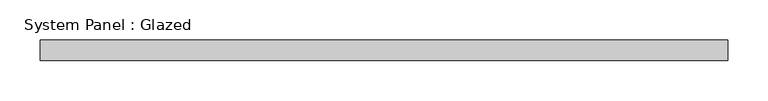
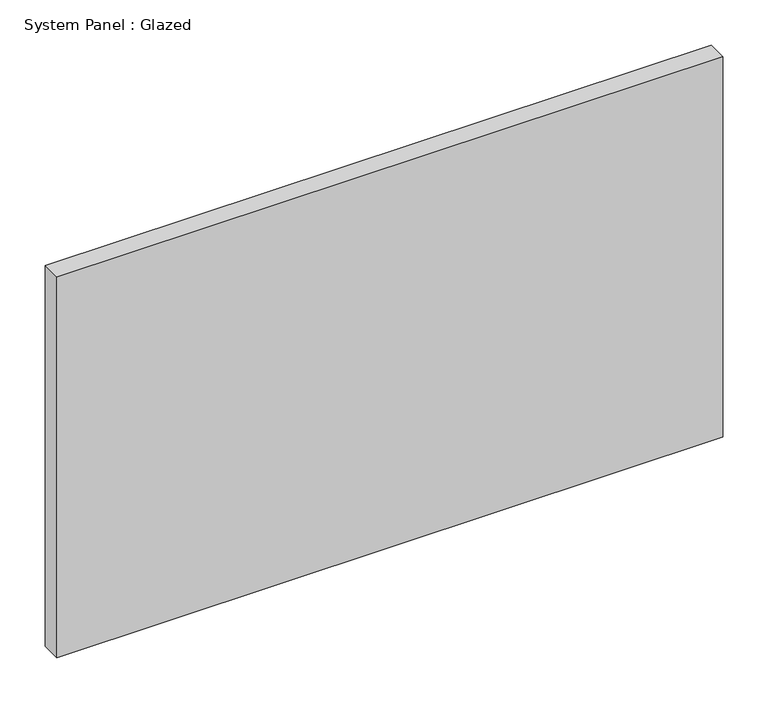
"""IFC4 building model written with IfcOpenShell, lengths in millimetres: plate geometry, System Panel : Glazed."""

from ifc_helpers import new_model, si_unit, origin, origin_with_axes, place, context, project, spatial, polyline, outline, extrude, source, transform, mapped, element, save


def system_panel_glazed_34036fae(model_context):
    return source(origin(), model_context, "Body", "SweptSolid", [
        extrude(outline(polyline([(425.45, -44.45), (-425.45, -44.45), (-425.45, -19.05), (425.45, -19.05), (425.45, -44.45)])), origin_with_axes(), (0.0, 0.0, 1.0), 514.35),
    ])


if __name__ == "__main__":
    model = new_model("IFC4")
    model_context = context("Model", 3, world=origin())
    ifc_project = project(units=[si_unit("LENGTHUNIT", "METRE", prefix="MILLI")], contexts=[model_context])
    site = spatial("IfcSite", under=ifc_project)
    building = spatial("IfcBuilding", under=site)
    placement = place(None, origin())
    system_panel_glazed_shape = system_panel_glazed_34036fae(model_context)
    element("IfcPlate", 1, ObjectType="System Panel : Glazed", at=placement, inside=building, context=model_context, shape_type="MappedRepresentation", body=[
        mapped(system_panel_glazed_shape, transform((0.0, 0.0, 0.0), x_axis=(1.0, 0.0, 0.0), y_axis=(0.0, 1.0, 0.0), z_axis=(0.0, 0.0, 1.0))),
    ])
    save(model, "model.ifc")

# Revit data of these elements
# Type "System Panel : Glazed"
#   Construction Type Id = "GSP4R"
#   Analytic Construction = "1/8 in Pilkington single glazing"
#   Visual Light Transmittance = 0.9
#   Solar Heat Gain Coefficient = 0.86
#   Heat Transfer Coefficient (U) = 1.18115 BTU/(h·ft²·°F)
# Element 1 (IfcPlate, "System Panel : Glazed")
#   Materials on its faces: "Glass"
# Materials
#   "Glass": class "Glass", colour RGB 0 128 192, transparency 0.75, Description = "Soda Lime Glass", Cost = 0
